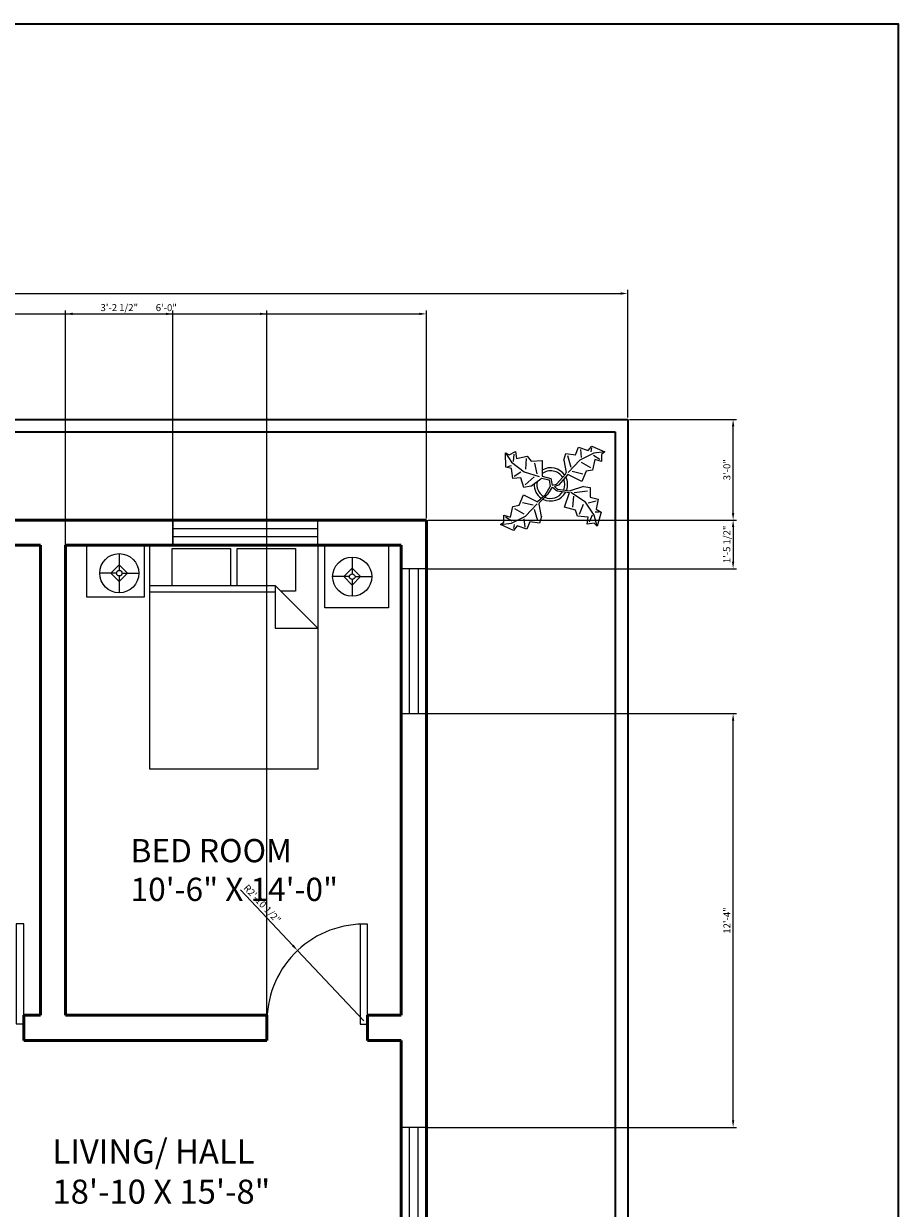
# Model space of a CAD drawing. Units: inches. Extents: x 65 to 818, y -87 to 880.
# Tile 6 of 6: x 505 to 818, y 457 to 880. Entities that reach past the tile are written whole.
import ezdxf

# ---------------------------------------------------------------- set-up
doc = ezdxf.new("R2010")
doc.units = ezdxf.units.IN
for name, color, linetype, lineweight in [('A-ANNO-DIMS', 2, 'Continuous', 18), ('A-ANNO-TTLB', 7, 'Continuous', 35), ('A-AREA-IDEN', 7, 'Continuous', 25), ('A-DOOR', 3, 'Continuous', 25), ('A-FURN', 8, 'Continuous', 18), ('A-GLAZ', 4, 'Continuous', 18), ('A-WALL', 7, 'Continuous', 50), ('C-PROP', 7, 'Continuous', 35), ('E-LITE', 2, 'Continuous', 18), ('L-PLNT', 94, 'Continuous', 13)]:
    doc.layers.add(name, color=color, linetype=linetype, lineweight=lineweight)
doc.styles.get("Standard").update_dxf_attribs({"font": 'arial.ttf'})
doc.dimstyles.new('ISO-25', dxfattribs={"dimtxt": 2.5, "dimasz": 2.5, "dimexe": 1.25, "dimexo": 0.625, "dimtad": 1, "dimtxsty": 'Standard', "dimcen": 2.5, "dimadec": 0, "dimazin": 0, "dimtfac": 1, "dimtmove": 0, "dimatfit": 3, "dimfxl": 1, "dimarcsym": 0})

# ---------------------------------------------------------------- blocks, each defined once
blk = doc.blocks.new('Bed - Queen')
for p, q in [((0, -80.00003), (0, 0)), ((0, 0), (59.99999, 0)), ((59.99999, 0), (59.99999, -80.00003)), ((7.99999, -1.2), (28.79998, -1.2)), ((7.99999, -14.4), (7.99999, -1.2)), ((28.79998, -1.2), (28.79998, -14.4)), ((31.19999, -1.2), (51.99999, -1.2)), ((31.19999, -14.4), (31.19999, -1.2)), ((51.99999, -1.2), (51.99999, -16.4)), ((0, -14.4), (44.8, -14.4)), ((44.8, -16.8), (0, -16.8)), ((59.99999, -29.6), (44.8, -14.4)), ((44.8, -14.4), (44.8, -29.6)), ((51.99999, -16.4), (46.79936, -16.4)), ((44.8, -29.6), (59.99999, -29.6)), ((59.99999, -80.00003), (0, -80.00003))]:
    blk.add_line(p, q)
blk = doc.blocks.new('Plant - Rubber or Philodendron')
for p, q in [((8.8871, 10.7908), (9.9809, 13.4933)), ((9.9809, 13.4933), (13.3837, 12.301)), ((13.3837, 12.301), (14.68, 13.9039)), ((14.5816, 13.2037), (14.3848, 11.8033)), ((14.68, 13.9039), (19.3848, 11.8146)), ((-16.2005, 11.4774), (-13.9899, 8.1064)), ((-16.2005, 11.4774), (-14.8639, 10.7964)), ((-16.0159, 6.3329), (-16.2005, 11.4774)), ((-14.8639, 10.7964), (-12.6195, 11.8975)), ((-13.3174, 8.325), (-13.0735, 11.0065)), ((-12.6195, 11.8975), (-12.1909, 9.4345)), ((-12.1909, 9.4345), (-8.3829, 10.3)), ((-8.8369, 9.409), (-9.0894, 5.6095)), ((-8.3829, 10.3), (-7.0549, 8.501)), ((-7.0549, 8.501), (-3.0284, 8.6941)), ((-3.0284, 8.6941), (-3.0709, 3.1041)), ((4.6914, 8.8812), (5.3859, 11.2828)), ((4.6914, 8.8812), (5.5014, 4.4831)), ((5.3859, 11.2828), (8.8871, 10.7908)), ((5.9878, 10.4842), (7.1971, 6.3869)), ((10.3916, 8.7942), (6.2847, 4.4028)), ((15.3859, 11.3055), (10.3916, 8.7942)), ((10.5828, 12.6946), (10.8893, 9.7953)), ((15.7909, 9.1065), (14.8995, 5.3044)), ((15.2875, 10.6053), (17.5907, 9.2105)), ((19.3848, 11.8146), (15.3859, 11.3055)), ((18.1925, 8.4119), (15.7909, 9.1065)), ((19.3848, 11.8146), (18.1868, 10.9119)), ((18.1868, 10.9119), (18.1925, 8.4119)), ((-14.0069, 5.8704), (-16.0159, 6.3329)), ((-15.3434, 6.5514), (-13.9984, 6.9884)), ((-13.5868, 2.2894), (-14.0069, 5.8704)), ((-13.9899, 8.1064), (-9.5434, 4.7185)), ((-13.1329, 3.1804), (-10.6614, 4.727)), ((-9.5434, 4.7185), (-4.1917, 2.9888)), ((-4.8529, 4.012), (-5.7184, 7.82)), ((5.4346, 3.9146), (5.5014, 4.4831)), ((7.7005, 4.8881), (11.5025, 3.9967)), ((14.2977, 6.1031), (10.9934, 7.9956)), ((12.7005, 4.8994), (11.1089, 1.1958)), ((14.8995, 5.3044), (12.7005, 4.8994)), ((-10.6784, 2.491), (-13.5868, 2.2894)), ((-9.5858, -0.8715), (-10.6784, 2.491)), ((-9.1318, 0.0195), (-5.9793, 2.9025)), ((-7.1228, -0.443), (-3.5248, 2.2131)), ((-3.5248, 2.2131), (-3.3011, 2.4355)), ((-3.3011, 2.4355), (-0.5306, 1.7947)), ((-3.0709, 3.1041), (0.0797, 2.3163)), ((-0.5306, 1.7947), (-0.2255, -0.5527)), ((-0.5306, 1.7947), (-0.5306, 1.7947)), ((0.0797, 2.3163), (0.4866, -0.031)), ((0.4866, -0.031), (2.1141, 0.2298)), ((2.1141, 0.2298), (5.4346, 3.9146)), ((6.1032, 3.6844), (2.8262, -0.031)), ((11.1089, 1.1958), (6.1032, 3.6844)), ((-11.3237, -7.2629), (-9.7321, -3.5593)), ((-9.7321, -3.5593), (-4.7264, -6.0479)), ((-7.1228, -0.443), (-9.5858, -0.8715)), ((-2.019, -3.6148), (-4.7264, -6.0479)), ((-4.0579, -6.2781), (-0.9375, -3.1608)), ((-2.019, -3.6148), (-0.2255, -0.5527)), ((-0.9375, -3.1608), (0.5883, -0.8135)), ((0.5883, -0.8135), (2.2447, -2.0916)), ((2.8262, -0.031), (1.3003, -0.5527)), ((1.3003, -0.5527), (2.4193, -1.4655)), ((2.2447, -2.0916), (6.7108, -2.6626)), ((2.4193, -1.4655), (6.895, -2.1175)), ((4.943, -7.9659), (6.7108, -2.6626)), ((11.6605, -0.5413), (6.895, -2.1175)), ((12.3677, -6.1981), (7.219, -2.6772)), ((8.125, -4.0768), (7.7715, -7.9659)), ((8.3544, -2.7453), (13.1973, -2.1704)), ((11.6605, -0.5413), (14.1354, -0.8948)), ((14.1354, -0.8948), (14.1354, -4.4304)), ((-14.4141, -11.4699), (-13.5228, -7.6679)), ((-13.5228, -7.6679), (-11.3237, -7.2629)), ((-12.921, -8.4665), (-9.6166, -10.359)), ((-6.3237, -7.2516), (-10.1257, -6.3602)), ((-9.0148, -11.1577), (-4.9047, -6.8122)), ((-4.1246, -6.8466), (-4.0579, -6.2781)), ((-3.3146, -11.2447), (-4.1246, -6.8466)), ((8.8321, -9.0266), (4.943, -7.9659)), ((10.2463, -10.4408), (11.6605, -6.9053)), ((15.5496, -10.7943), (12.3677, -6.1981)), ((16.2567, -5.8446), (13.4283, -6.5517)), ((14.1354, -4.4304), (16.9638, -5.1375)), ((16.9638, -5.1375), (16.2567, -8.673)), ((-16.8157, -10.7754), (-14.4141, -11.4699)), ((-16.8101, -13.2754), (-16.8157, -10.7754)), ((-13.9107, -12.9688), (-16.2139, -11.574)), ((-14.0091, -13.669), (-9.0148, -11.1577)), ((-9.206, -15.0581), (-9.5126, -12.1588)), ((-4.611, -12.8477), (-5.8203, -8.7504)), ((-3.3146, -11.2447), (-4.0092, -13.6463)), ((9.5392, -11.1479), (8.8321, -9.0266)), ((13.4283, -11.5015), (9.5392, -11.1479)), ((13.0748, -13.9763), (13.4283, -11.5015)), ((14.8425, -10.7943), (13.7819, -13.2692)), ((16.6103, -14.6834), (15.5496, -10.7943)), ((17.3174, -9.7337), (15.9032, -9.7337)), ((16.2567, -8.673), (18.0245, -9.7337)), ((18.0245, -9.7337), (16.6103, -14.6834)), ((-18.008, -14.1781), (-16.8101, -13.2754)), ((-18.008, -14.1781), (-14.0091, -13.669)), ((-13.3032, -16.2674), (-18.008, -14.1781)), ((-12.0069, -14.6645), (-13.3032, -16.2674)), ((-13.2048, -15.5672), (-13.008, -14.1668)), ((-8.6042, -15.8568), (-12.0069, -14.6645)), ((-7.5103, -13.1543), (-8.6042, -15.8568)), ((-4.0092, -13.6463), (-7.5103, -13.1543)), ((15.5496, -13.6228), (13.0748, -13.9763)), ((16.6103, -14.6834), (15.5496, -13.6228))]:
    blk.add_line(p, q)
for centre, radius, start, end in [((0, 0), 6.1275, 34.37569, 120.1028), ((-0.0601, -0.2075), 5.2461, 33.82192, 124.9414), ((0.0308, 0.1664), 6, 178.6147, 235.1169), ((0.0308, 0.1664), 5, 168.1647, 238.6725), ((-0.2664, 0.1682), 5.2775, 338.4094, 20.03007), ((-0.098, 0.1364), 6.1288, 341.2017, 26.09184), ((-0.0234, 0.3825), 6.1492, 242.5812, 331.2714), ((-0.1102, 0.4886), 5.2883, 247.3711, 327.472)]:
    blk.add_arc(centre, radius, start, end)
blk = doc.blocks.new('Lamp - Table')
for p, q in [((0, 7), (0, 1)), ((-1, 0), (-7, 0)), ((0, 3), (-3, 0)), ((-3, 0), (0, -3)), ((3, 0), (0, 3)), ((0, -3), (3, 0)), ((1, 0), (7, 0)), ((0, -1), (0, -7))]:
    blk.add_line(p, q)
for radius in [7, 1]:
    blk.add_circle((0, 0), radius)
blk = doc.blocks.new('*D13')
at = {"layer": 'A-ANNO-DIMS', "color": 0, "lineweight": -2, "transparency": 16777216}
for p, q in [((240.8, 739.67), (240.8, 785.28)), ((243.3, 784.03), (718.3, 784.03)), ((720.8, 739.67), (720.8, 785.28))]:
    blk.add_line(p, q, dxfattribs=at)
at = {"layer": 'A-ANNO-DIMS', "color": 0, "transparency": 16777216}
for points in [[(243.3, 784.45), (243.3, 783.61), (240.8, 784.03)], [(718.3, 784.45), (718.3, 783.61), (720.8, 784.03)]]:
    blk.add_solid(points, dxfattribs=at)
at = {"layer": 'Defpoints', "color": 0, "transparency": 16777216}
for p in [(720.8, 784.03), (240.8, 739.04), (720.8, 739.04)]:
    blk.add_point(p, dxfattribs=at)
at = {"layer": 'A-ANNO-DIMS', "color": 0, "transparency": 16777216, "insert": (480.8, 785.17), "char_height": 1, "attachment_point": 5}
blk.add_mtext("40'", dxfattribs=at)
blk = doc.blocks.new('WIN-52X9-PLAN')
for p, q in [((9, 51.82), (0, 51.82)), ((0, 51.82), (0, 0)), ((3, 0), (3, 51.82)), ((6, 51.82), (6, 0)), ((9, 0), (9, 51.82)), ((0, 0), (9, 0))]:
    blk.add_line(p, q)
blk = doc.blocks.new('DOOR-LEAF-36-NOM')
blk.add_lwpolyline([(0, 0), (2.67, 0), (2.67, 35.67), (0, 35.67)], close=True)
blk = doc.blocks.new('*D49')
at = {"layer": 'A-ANNO-DIMS', "color": 0, "lineweight": -2, "transparency": 16777216}
for p, q in [((519.8, 526.67), (519.8, 777.99)), ((522.3, 776.74), (589.3, 776.74)), ((591.8, 526.67), (591.8, 777.99))]:
    blk.add_line(p, q, dxfattribs=at)
at = {"layer": 'A-ANNO-DIMS', "color": 0, "transparency": 16777216}
for points in [[(522.3, 777.16), (522.3, 776.32), (519.8, 776.74)], [(589.3, 777.16), (589.3, 776.32), (591.8, 776.74)]]:
    blk.add_solid(points, dxfattribs=at)
at = {"layer": 'Defpoints', "color": 0, "transparency": 16777216}
for p in [(591.8, 776.74), (519.8, 526.04), (591.8, 526.04)]:
    blk.add_point(p, dxfattribs=at)
at = {"layer": 'A-ANNO-DIMS', "color": 0, "transparency": 16777216, "insert": (555.8, 778.64), "char_height": 2.5, "attachment_point": 5}
blk.add_mtext('6\'-0"', dxfattribs=at)
blk = doc.blocks.new('*D50')
at = {"layer": 'A-ANNO-DIMS', "color": 0, "lineweight": -2, "transparency": 16777216}
for p, q in [((240.8, 703.67), (240.8, 777.99)), ((243.3, 776.74), (646.3, 776.74)), ((648.8, 703.67), (648.8, 777.99))]:
    blk.add_line(p, q, dxfattribs=at)
at = {"layer": 'A-ANNO-DIMS', "color": 0, "transparency": 16777216}
for points in [[(243.3, 777.16), (243.3, 776.32), (240.8, 776.74)], [(646.3, 777.16), (646.3, 776.32), (648.8, 776.74)]]:
    blk.add_solid(points, dxfattribs=at)
at = {"layer": 'Defpoints', "color": 0, "transparency": 16777216}
for p in [(648.8, 776.74), (240.8, 703.04), (648.8, 703.04)]:
    blk.add_point(p, dxfattribs=at)
at = {"layer": 'A-ANNO-DIMS', "color": 0, "transparency": 16777216, "insert": (444.8, 778.64), "char_height": 2.5, "attachment_point": 5}
blk.add_mtext('34\'-0"', dxfattribs=at)
blk = doc.blocks.new('*D51')
at = {"layer": 'A-ANNO-DIMS', "color": 0, "lineweight": -2, "transparency": 16777216}
for p, q in [((721.42, 739.04), (759.75, 739.04)), ((758.5, 705.54), (758.5, 736.54)), ((649.42, 703.04), (759.75, 703.04))]:
    blk.add_line(p, q, dxfattribs=at)
at = {"layer": 'A-ANNO-DIMS', "color": 0, "transparency": 16777216}
for points in [[(758.08, 736.54), (758.92, 736.54), (758.5, 739.04)], [(758.08, 705.54), (758.92, 705.54), (758.5, 703.04)]]:
    blk.add_solid(points, dxfattribs=at)
at = {"layer": 'Defpoints', "color": 0, "transparency": 16777216}
for p in [(720.8, 739.04), (758.5, 739.04), (648.8, 703.04)]:
    blk.add_point(p, dxfattribs=at)
at = {"layer": 'A-ANNO-DIMS', "color": 0, "transparency": 16777216, "insert": (756.6, 721.04), "char_height": 2.5, "attachment_point": 5, "rotation": 90}
blk.add_mtext('3\'-0"', dxfattribs=at)
blk = doc.blocks.new('*D59')
at = {"layer": 'A-ANNO-DIMS', "color": 0, "lineweight": -2, "transparency": 16777216}
for p, q in [((649.42, 703.04), (759.75, 703.04)), ((758.5, 700.54), (758.5, 688.16)), ((649.44, 685.66), (759.75, 685.66))]:
    blk.add_line(p, q, dxfattribs=at)
at = {"layer": 'A-ANNO-DIMS', "color": 0, "transparency": 16777216}
for points in [[(758.08, 700.54), (758.92, 700.54), (758.5, 703.04)], [(758.08, 688.16), (758.92, 688.16), (758.5, 685.66)]]:
    blk.add_solid(points, dxfattribs=at)
at = {"layer": 'Defpoints', "color": 0, "transparency": 16777216}
for p in [(648.8, 703.04), (648.82, 685.66), (758.5, 685.66)]:
    blk.add_point(p, dxfattribs=at)
at = {"layer": 'A-ANNO-DIMS', "color": 0, "transparency": 16777216, "insert": (756.58, 694.35), "char_height": 2.5, "attachment_point": 5, "rotation": 90}
blk.add_mtext('1\'-5 1/2"', dxfattribs=at)
blk = doc.blocks.new('*D63')
at = {"layer": 'A-ANNO-DIMS', "color": 0, "lineweight": -2, "transparency": 16777216}
for p, q in [((519.8, 694.67), (519.8, 777.99)), ((522.3, 776.74), (555.68, 776.74)), ((558.18, 694.65), (558.18, 777.99))]:
    blk.add_line(p, q, dxfattribs=at)
at = {"layer": 'A-ANNO-DIMS', "color": 0, "transparency": 16777216}
for points in [[(522.3, 777.16), (522.3, 776.32), (519.8, 776.74)], [(555.68, 777.16), (555.68, 776.32), (558.18, 776.74)]]:
    blk.add_solid(points, dxfattribs=at)
at = {"layer": 'Defpoints', "color": 0, "transparency": 16777216}
for p in [(558.18, 776.74), (519.8, 694.04), (558.18, 694.03)]:
    blk.add_point(p, dxfattribs=at)
at = {"layer": 'A-ANNO-DIMS', "color": 0, "transparency": 16777216, "insert": (538.99, 778.66), "char_height": 2.5, "attachment_point": 5}
blk.add_mtext('3\'-2 1/2"', dxfattribs=at)
blk = doc.blocks.new('*D67')
at = {"layer": 'A-ANNO-DIMS', "color": 0, "lineweight": -2, "transparency": 16777216}
for p, q in [((649.44, 633.84), (759.75, 633.84)), ((758.5, 488.46), (758.5, 631.34)), ((649.42, 485.96), (759.75, 485.96))]:
    blk.add_line(p, q, dxfattribs=at)
at = {"layer": 'A-ANNO-DIMS', "color": 0, "transparency": 16777216}
for points in [[(758.08, 631.34), (758.92, 631.34), (758.5, 633.84)], [(758.08, 488.46), (758.92, 488.46), (758.5, 485.96)]]:
    blk.add_solid(points, dxfattribs=at)
at = {"layer": 'Defpoints', "color": 0, "transparency": 16777216}
for p in [(648.82, 633.84), (758.5, 633.84), (648.8, 485.96)]:
    blk.add_point(p, dxfattribs=at)
at = {"layer": 'A-ANNO-DIMS', "color": 0, "transparency": 16777216, "insert": (756.62, 559.9), "char_height": 2.5, "attachment_point": 5, "rotation": 90}
blk.add_mtext('12\'-4"', dxfattribs=at)
blk = doc.blocks.new('*D77')
at = {"layer": 'A-ANNO-DIMS', "color": 0, "lineweight": -2, "transparency": 16777216}
for p, q in [((582.31, 570.89), (601.01, 551.01)), ((626.44, 523.99), (602.72, 549.19))]:
    blk.add_line(p, q, dxfattribs=at)
at = {"layer": 'A-ANNO-DIMS', "color": 0, "transparency": 16777216}
blk.add_solid([(601.31, 551.3), (600.7, 550.73), (602.72, 549.19)], dxfattribs=at)
at = {"layer": 'Defpoints', "color": 0, "transparency": 16777216}
for p in [(602.72, 549.19), (626.44, 523.99)]:
    blk.add_point(p, dxfattribs=at)
at = {"layer": 'A-ANNO-DIMS', "color": 0, "transparency": 16777216, "insert": (589.89, 565.63), "char_height": 2.5, "attachment_point": 5, "rotation": 313.2558}
blk.add_mtext('R2\'-10 1/2"', dxfattribs=at)

msp = doc.modelspace()

# ---------------------------------------------------------------- linework, layer by layer
at = {"layer": 'A-ANNO-TTLB'}
msp.add_lwpolyline([(64.55, 880.46), (817.59, 880.46), (817.59, -87.37), (64.55, -87.37)], close=True, dxfattribs=at)
at = {"layer": 'A-DOOR'}
msp.add_arc((626.44, 523.99), 34.61, 87.7499, 178.7625, dxfattribs=at)
at = {"layer": 'A-FURN'}
for points in [[(527.38, 694), (547.88, 694), (547.88, 675.52), (527.38, 675.52)], [(612.54, 693.96), (635.32, 693.96), (635.32, 671.62), (612.54, 671.62)]]:
    msp.add_lwpolyline(points, close=True, dxfattribs=at)
at = {"layer": 'A-WALL'}
for p, q in [((240.8, 703.04), (648.8, 703.04)), ((648.8, 703.04), (648.8, 138.54)), ((342.8, 694.04), (510.8, 694.04)), ((510.8, 526.04), (510.8, 694.04)), ((519.8, 526.04), (519.8, 694.04)), ((519.8, 694.04), (639.8, 694.04)), ((639.8, 694.04), (639.8, 526.04)), ((504.8, 517.04), (504.8, 526.04)), ((504.8, 526.04), (510.8, 526.04)), ((519.8, 526.04), (591.8, 526.04)), ((591.8, 526.04), (591.8, 517.04)), ((627.8, 526.04), (627.8, 517.04)), ((627.8, 526.04), (639.8, 526.04)), ((504.8, 517.04), (591.8, 517.04)), ((504.8, 517.04), (591.8, 517.04)), ((627.8, 517.04), (639.8, 517.04)), ((627.8, 517.04), (639.8, 517.04)), ((639.8, 517.04), (639.8, 429.07))]:
    msp.add_line(p, q, dxfattribs=at)
at = {"layer": 'C-PROP'}
for p, q in [((240.8, 739.04), (720.8, 739.04)), ((720.8, 739.04), (720.8, 451.35)), ((240.8, 734.54), (716.3, 734.54)), ((716.3, 734.54), (716.3, 23.54))]:
    msp.add_line(p, q, dxfattribs=at)

# ---------------------------------------------------------------- block references
at = {"layer": 'A-DOOR'}
for p in [(502.13, 523), (625.13, 522.9)]:
    msp.add_blockref('DOOR-LEAF-36-NOM', p, dxfattribs=at)
at = {"layer": 'A-FURN'}
msp.add_blockref('Bed - Queen', (549.95, 694.05), dxfattribs=at)
at = {"layer": 'A-GLAZ'}
for p, rotation in [((558.18, 703.03), 270.0000000000001), ((648.82, 685.66), 180)]:
    msp.add_blockref('WIN-52X9-PLAN', p, dxfattribs=dict(at, rotation=rotation))
msp.add_blockref('WIN-52X9-PLAN', (639.8, 434.13), dxfattribs=at)
at = {"layer": 'E-LITE'}
for p in [(538.98, 684.05), (622.29, 682.81)]:
    msp.add_blockref('Lamp - Table', p, dxfattribs=at)
at = {"layer": 'L-PLNT'}
msp.add_blockref('Plant - Rubber or Philodendron', (693.29, 715.6), dxfattribs=at)

# ---------------------------------------------------------------- texts
at = {"layer": 'A-AREA-IDEN', "attachment_point": 1}
for s, width, gutter_width, insert, char_height in [('BED ROOM \\P10\'-6" X 14\'-0"', 175.5324, 41.53, (543.03, 589.03), 8.305), ('LIVING/ HALL\\P18\'-10 X 15\'-8"', 370.469, 43.06, (515.08, 481.64), 8.612)]:
    msp.add_mtext_dynamic_manual_height_columns(s, width=width, gutter_width=gutter_width, heights=[0], dxfattribs=dict(at, insert=insert, char_height=char_height))

# ---------------------------------------------------------------- dimensions: what is measured, and where the dimension line sits
at = {"layer": 'A-ANNO-DIMS'}
for base, p1, p2, override, picture, middle in [((720.8, 784.03), (240.8, 739.04), (720.8, 739.04), {"dimtxt": 1, "dimdec": 0, "dimlunit": 3, "dimclrd": 0, "dimclre": 0, "dimclrt": 0, "dimtdec": 0}, '*D13', (480.8, 785.17)), ((648.8, 776.74), (240.8, 703.04), (648.8, 703.04), {"dimdec": 1, "dimlfac": 1, "dimrnd": 0, "dimzin": 1, "dimdsep": 46, "dimlunit": 4, "dimfrac": 2}, '*D50', (444.8, 778.64)), ((558.18, 776.74), (519.8, 694.04), (558.18, 694.03), {"dimdec": 1, "dimlfac": 1, "dimrnd": 0, "dimzin": 1, "dimdsep": 46, "dimlunit": 4, "dimfrac": 2}, '*D63', (538.99, 778.66)), ((591.8, 776.74), (519.8, 526.04), (591.8, 526.04), {"dimdec": 1, "dimlfac": 1, "dimrnd": 0, "dimzin": 1, "dimdsep": 46, "dimlunit": 4, "dimfrac": 2}, '*D49', (555.8, 778.64))]:
    dim = msp.add_linear_dim(base=base, p1=p1, p2=p2, dimstyle='ISO-25', override=override, dxfattribs=at)
    dim.commit()
    dim.dimension.update_dxf_attribs({"geometry": picture, "text_midpoint": middle})
for base, p1, p2, picture, middle in [((758.5, 739.04), (648.8, 703.04), (720.8, 739.04), '*D51', (756.6, 721.04)), ((758.5, 685.66), (648.8, 703.04), (648.82, 685.66), '*D59', (756.58, 694.35)), ((758.5, 633.84), (648.8, 485.96), (648.82, 633.84), '*D67', (756.62, 559.9))]:
    dim = msp.add_linear_dim(base=base, p1=p1, p2=p2, angle=90, dimstyle='ISO-25', override={"dimdec": 1, "dimlfac": 1, "dimrnd": 0, "dimzin": 1, "dimdsep": 46, "dimlunit": 4, "dimfrac": 2}, dxfattribs=at)
    dim.commit()
    dim.dimension.update_dxf_attribs({"geometry": picture, "text_midpoint": middle})
dim = msp.add_radius_dim(center=(626.44, 523.99), mpoint=(602.72, 549.19), dimstyle='ISO-25', override={"dimdec": 1, "dimlfac": 1, "dimrnd": 0, "dimzin": 1, "dimdsep": 46, "dimlunit": 4, "dimfrac": 2}, dxfattribs=at)
dim.commit()
dim.dimension.update_dxf_attribs({"geometry": '*D77', "text_midpoint": (588.49, 564.32), "dimtype": 164})

doc.saveas('drawing.dxf')
